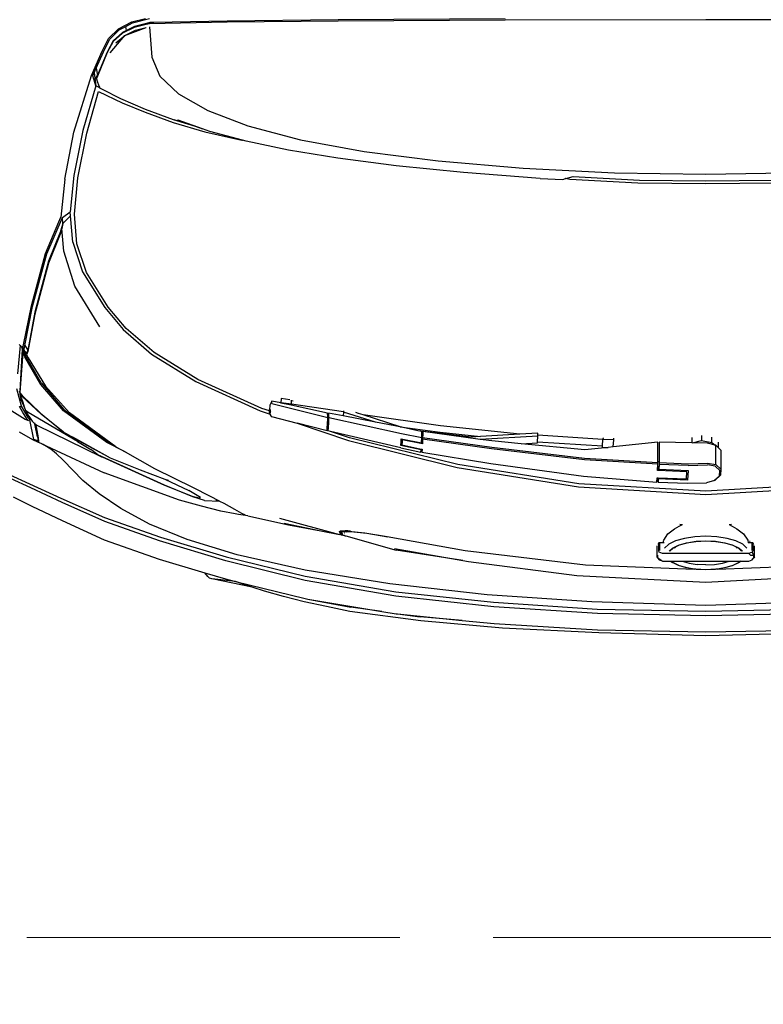
# Model space of a CAD drawing. Units: inches. Extents: x 0 to 4258, y 0 to 3769.
# Tile 6 of 30: x 3739 to 3762, y 2971 to 3003. Entities that reach past the tile are written whole.
import ezdxf

# ---------------------------------------------------------------- set-up
doc = ezdxf.new("R2010")
doc.units = ezdxf.units.IN
doc.header["$MEASUREMENT"] = 0
doc.linetypes.add('ACAD_ISO02W100', pattern=[15, 12, -3])
doc.layers.get('0').update_dxf_attribs({"color": 16})
for name, color, linetype, lineweight in [('A-ANNO-DIMS', 250, 'Continuous', 18), ('A-FLOR-OVHD', 150, 'ACAD_ISO02W100', 13), ('C-PKNG-VEHI', 8, 'Continuous', 18)]:
    doc.layers.add(name, color=color, linetype=linetype, lineweight=lineweight)
doc.layers.add('Edges', color=250, linetype='Continuous')
doc.styles.get("Standard").update_dxf_attribs({"font": 'arial.ttf'})
doc.dimstyles.get("Standard").update_dxf_attribs({"dimtxt": 7, "dimasz": 0.18, "dimexe": 0.18, "dimexo": 0.0625, "dimgap": 0.09, "dimtad": 0, "dimtih": 1, "dimtoh": 1, "dimzin": 0, "dimdsep": 46, "dimlunit": 3, "dimtxsty": 'Standard', "dimcen": 0.09, "dimadec": 0, "dimazin": 0, "dimtfac": 1, "dimtofl": 0, "dimtmove": 0, "dimatfit": 3, "dimfxl": 1, "dimtolj": 1, "dimtzin": 0, "dimarcsym": 0})

# ---------------------------------------------------------------- blocks, each defined once
blk = doc.blocks.new('Nissan Qashqai pl')
at = {"layer": 'Edges'}
for p, q in [((11.05972, 12.11965), (11.05938, 11.92208)), ((11.61327, 11.92208), (11.60675, 12.04892)), ((11.5166, 12.04708), (11.52386, 11.92208)), ((11.52698, 11.92208), (11.51964, 12.0475)), ((11.60051, 11.93346), (11.59629, 12.04057)), ((11.63292, 12.0344), (11.63628, 11.92208)), ((11.64211, 11.92208), (11.63993, 12.02899)), ((11.64437, 12.02886), (11.64655, 11.92208)), ((11.66226, 11.92208), (11.66041, 12.02874)), ((11.66349, 12.02738), (11.66628, 11.92208)), ((11.21164, 11.92208), (11.21014, 12.01197)), ((11.21801, 11.92208), (11.21745, 11.98742)), ((11.22044, 11.98904), (11.22108, 11.92208)), ((11.58846, 11.97008), (11.57758, 11.97008)), ((11.58846, 11.97008), (11.58961, 11.96947)), ((11.56588, 11.95938), (11.57195, 11.96347)), ((11.57195, 11.96347), (11.57457, 11.96395)), ((11.57261, 11.96533), (11.57261, 11.96561)), ((11.57306, 11.96528), (11.57306, 11.96569)), ((11.57479, 11.96843), (11.57457, 11.96768)), ((11.58239, 11.96768), (11.57457, 11.96768)), ((11.57457, 11.96768), (11.57457, 11.96395)), ((11.57457, 11.96395), (11.57457, 11.96378)), ((11.57617, 11.96938), (11.57479, 11.96843)), ((11.57479, 11.96843), (11.58262, 11.96843)), ((11.57994, 11.96265), (11.57613, 11.95845)), ((11.58262, 11.96843), (11.58377, 11.96782)), ((11.58668, 11.96947), (11.58377, 11.96782)), ((11.58377, 11.96782), (11.58513, 11.96453)), ((11.58679, 11.96604), (11.58513, 11.96453)), ((11.58513, 11.96453), (11.58513, 11.87963)), ((11.58679, 11.96604), (11.58668, 11.96947)), ((11.58961, 11.96947), (11.58668, 11.96947)), ((11.5915, 11.96782), (11.58961, 11.96947)), ((11.5915, 11.96782), (11.59043, 11.96839)), ((11.59285, 11.96453), (11.5915, 11.96782)), ((11.59285, 11.95694), (11.59285, 11.96453)), ((11.55816, 11.94815), (11.56082, 11.95281)), ((11.56082, 11.95281), (11.56588, 11.95938)), ((11.57286, 11.95178), (11.57035, 11.94308)), ((11.57613, 11.95845), (11.57286, 11.95178)), ((11.57692, 11.94885), (11.57987, 11.95487)), ((11.57876, 11.95169), (11.57712, 11.94834)), ((11.58001, 11.95424), (11.57876, 11.95169)), ((11.57876, 11.95169), (11.57995, 11.953)), ((11.57987, 11.95487), (11.58291, 11.95821)), ((11.58291, 11.95743), (11.58001, 11.95424)), ((11.59285, 11.95694), (11.59412, 11.95487)), ((11.59285, 11.95657), (11.59285, 11.95694)), ((11.59319, 11.9559), (11.59285, 11.95657)), ((11.59285, 11.95626), (11.59285, 11.95657)), ((11.59285, 11.95626), (11.59319, 11.9559)), ((11.59285, 11.95549), (11.59285, 11.95626)), ((11.59398, 11.95424), (11.59285, 11.95549)), ((11.59285, 11.94526), (11.59285, 11.95549)), ((11.59319, 11.9559), (11.59412, 11.95487)), ((11.59688, 11.94834), (11.59398, 11.95424)), ((11.59412, 11.95487), (11.59707, 11.94885)), ((11.55654, 11.94509), (11.55639, 11.94749)), ((11.55654, 11.94509), (11.55816, 11.94815)), ((11.57035, 11.94308), (11.56877, 11.93295)), ((11.57324, 11.93188), (11.57466, 11.94101)), ((11.57466, 11.94101), (11.57692, 11.94885)), ((11.57712, 11.94834), (11.5749, 11.94065)), ((11.59285, 11.8989), (11.59285, 11.94526)), ((11.59478, 11.93858), (11.59285, 11.94526)), ((11.5991, 11.94065), (11.59688, 11.94834)), ((11.59707, 11.94885), (11.59933, 11.94101)), ((11.59933, 11.94101), (11.60051, 11.93346)), ((11.48106, 11.93457), (11.47554, 11.93456)), ((11.47578, 11.92803), (11.4784, 11.93124)), ((11.4784, 11.93124), (11.47657, 11.92368)), ((11.4786, 11.93206), (11.4784, 11.93124)), ((11.48106, 11.93457), (11.4786, 11.93206)), ((11.49744, 11.93207), (11.4786, 11.93206)), ((11.48349, 11.93703), (11.48106, 11.93457)), ((11.48349, 11.93703), (11.50222, 11.93704)), ((11.49621, 11.92369), (11.49744, 11.93207)), ((11.49744, 11.93207), (11.50222, 11.93704)), ((11.49907, 11.93132), (11.49795, 11.92364)), ((11.50349, 11.93588), (11.49907, 11.93132)), ((11.50222, 11.93704), (11.50812, 11.93671)), ((11.50889, 11.93558), (11.50349, 11.93588)), ((11.50812, 11.93671), (11.51287, 11.9312)), ((11.50889, 11.93558), (11.51321, 11.93053)), ((11.51321, 11.93053), (11.51287, 11.9312)), ((11.56877, 11.93295), (11.56823, 11.92208)), ((11.57275, 11.92208), (11.57324, 11.93188)), ((11.5735, 11.93169), (11.57302, 11.92208)), ((11.5749, 11.94065), (11.5735, 11.93169)), ((11.59602, 11.93062), (11.59478, 11.93858)), ((11.60049, 11.93169), (11.5991, 11.94065)), ((11.60097, 11.92208), (11.60049, 11.93169)), ((11.60051, 11.93346), (11.60076, 11.93188)), ((11.60076, 11.93188), (11.60124, 11.92208)), ((11.05938, 11.92208), (11.05972, 11.72451)), ((11.21014, 11.8322), (11.21164, 11.92208)), ((11.21745, 11.85674), (11.21801, 11.92208)), ((11.22108, 11.92208), (11.22044, 11.85512)), ((11.47578, 11.92803), (11.47062, 11.92803)), ((11.47398, 11.91798), (11.47578, 11.92803)), ((11.47657, 11.92368), (11.47622, 11.90912)), ((11.49689, 11.90495), (11.49621, 11.92369)), ((11.49859, 11.9049), (11.49795, 11.92364)), ((11.51321, 11.93053), (11.51543, 11.92267)), ((11.51606, 11.90392), (11.51543, 11.92267)), ((11.52386, 11.92208), (11.5166, 11.79708)), ((11.51964, 11.79666), (11.52698, 11.92208)), ((11.56823, 11.92208), (11.56877, 11.91121)), ((11.57324, 11.91228), (11.57275, 11.92208)), ((11.57302, 11.92208), (11.5735, 11.91247)), ((11.59645, 11.92208), (11.59602, 11.93062)), ((11.59645, 11.92208), (11.59602, 11.91354)), ((11.60049, 11.91247), (11.60097, 11.92208)), ((11.60124, 11.92208), (11.60076, 11.91228)), ((11.60675, 11.79524), (11.61327, 11.92208)), ((11.63628, 11.92208), (11.63292, 11.80976)), ((11.63993, 11.81518), (11.64211, 11.92208)), ((11.64655, 11.92208), (11.64437, 11.8153)), ((11.66041, 11.81542), (11.66226, 11.92208)), ((11.66628, 11.92208), (11.66349, 11.81678)), ((11.46896, 11.91798), (11.47398, 11.91798)), ((11.47622, 11.90912), (11.47398, 11.91798)), ((11.57466, 11.90315), (11.57324, 11.91228)), ((11.5735, 11.91247), (11.5749, 11.90351)), ((11.59478, 11.90558), (11.59602, 11.91354)), ((11.5991, 11.90351), (11.60049, 11.91247)), ((11.60076, 11.91228), (11.60051, 11.91071)), ((11.47102, 11.90825), (11.4762, 11.90826)), ((11.4762, 11.90826), (11.47542, 11.87608)), ((11.47622, 11.90912), (11.4762, 11.90826)), ((11.49565, 11.87616), (11.49689, 11.90495)), ((11.49859, 11.9049), (11.49735, 11.87612)), ((11.50223, 11.8759), (11.50346, 11.90468)), ((11.50462, 11.90341), (11.50341, 11.87505)), ((11.50346, 11.90468), (11.51299, 11.90415)), ((11.51177, 11.90301), (11.50462, 11.90341)), ((11.51058, 11.87508), (11.51177, 11.90301)), ((11.51299, 11.90415), (11.51176, 11.87537)), ((11.51483, 11.87514), (11.51606, 11.90392)), ((11.56877, 11.91121), (11.57035, 11.90108)), ((11.57692, 11.89531), (11.57466, 11.90315)), ((11.5749, 11.90351), (11.57712, 11.89582)), ((11.59285, 11.8989), (11.59478, 11.90558)), ((11.59629, 11.80359), (11.60051, 11.91071)), ((11.59688, 11.89582), (11.5991, 11.90351)), ((11.59933, 11.90315), (11.59707, 11.89531)), ((11.60051, 11.91071), (11.59933, 11.90315)), ((11.55639, 11.89667), (11.55654, 11.89907)), ((11.55816, 11.89601), (11.55654, 11.89907)), ((11.56082, 11.89135), (11.55816, 11.89601)), ((11.57035, 11.90108), (11.57286, 11.89238)), ((11.57286, 11.89238), (11.57613, 11.88571)), ((11.57987, 11.88929), (11.57692, 11.89531)), ((11.57712, 11.89582), (11.57876, 11.89248)), ((11.57995, 11.89116), (11.57876, 11.89248)), ((11.57876, 11.89248), (11.58001, 11.88992)), ((11.59285, 11.88868), (11.59285, 11.8989)), ((11.59398, 11.88992), (11.59688, 11.89582)), ((11.59707, 11.89531), (11.59412, 11.88929)), ((11.56588, 11.88478), (11.56082, 11.89135)), ((11.57195, 11.88069), (11.56588, 11.88478)), ((11.57613, 11.88571), (11.57994, 11.88151)), ((11.58291, 11.88595), (11.57987, 11.88929)), ((11.58001, 11.88992), (11.58291, 11.88673)), ((11.59285, 11.88868), (11.59398, 11.88992)), ((11.59285, 11.88722), (11.59412, 11.88929)), ((11.59285, 11.8879), (11.59285, 11.88868)), ((11.59285, 11.88759), (11.59319, 11.88827)), ((11.59319, 11.88827), (11.59285, 11.8879)), ((11.59285, 11.88759), (11.59285, 11.8879)), ((11.59285, 11.88722), (11.59285, 11.88759)), ((11.59285, 11.87963), (11.59285, 11.88722)), ((11.59412, 11.88929), (11.59319, 11.88827)), ((11.49563, 11.87496), (11.47539, 11.87488)), ((11.47539, 11.87488), (11.4801, 11.83099)), ((11.47542, 11.87608), (11.49451, 11.87616)), ((11.49133, 11.80278), (11.49563, 11.87496)), ((11.49732, 11.87492), (11.49295, 11.80271)), ((11.49449, 11.87502), (11.49451, 11.87616)), ((11.50341, 11.87505), (11.49449, 11.87502)), ((11.49451, 11.87616), (11.49565, 11.87616)), ((11.49732, 11.87492), (11.49563, 11.87496)), ((11.49565, 11.87616), (11.49735, 11.87612)), ((11.50339, 11.87463), (11.49732, 11.87492)), ((11.49735, 11.87612), (11.50223, 11.8759)), ((11.50341, 11.87505), (11.50339, 11.87463)), ((11.50884, 11.80182), (11.5148, 11.87394)), ((11.51054, 11.87423), (11.51058, 11.87508)), ((11.5148, 11.87394), (11.51054, 11.87423)), ((11.51472, 11.8751), (11.51058, 11.87508)), ((11.51176, 11.87537), (11.51472, 11.87515)), ((11.51472, 11.87515), (11.51472, 11.8751)), ((11.51472, 11.87515), (11.51483, 11.87514)), ((11.51483, 11.87514), (11.51472, 11.8751)), ((11.57261, 11.88057), (11.57195, 11.88069)), ((11.57261, 11.88057), (11.57261, 11.88076)), ((11.57306, 11.88049), (11.57261, 11.88057)), ((11.57306, 11.88049), (11.57306, 11.88081)), ((11.57457, 11.88021), (11.57306, 11.88049)), ((11.57457, 11.88096), (11.57457, 11.88021)), ((11.57457, 11.88021), (11.57457, 11.87648)), ((11.57457, 11.87648), (11.58239, 11.87648)), ((11.57457, 11.87648), (11.57479, 11.87573)), ((11.58262, 11.87573), (11.57479, 11.87573)), ((11.57479, 11.87573), (11.57617, 11.87478)), ((11.58846, 11.87408), (11.57758, 11.87408)), ((11.58377, 11.87635), (11.58262, 11.87573)), ((11.58513, 11.87963), (11.58377, 11.87635)), ((11.58668, 11.87469), (11.58961, 11.87469)), ((11.58961, 11.87469), (11.58846, 11.87408)), ((11.58961, 11.87469), (11.5915, 11.87635)), ((11.59043, 11.87577), (11.58961, 11.87469)), ((11.59221, 11.87812), (11.59043, 11.87577)), ((11.59043, 11.87577), (11.5915, 11.87635)), ((11.5915, 11.87635), (11.59221, 11.87812)), ((11.59285, 11.87963), (11.59221, 11.87812)), ((11.2139, 11.7914), (11.21745, 11.85674)), ((11.22044, 11.85512), (11.21682, 11.78816)), ((11.20565, 11.74231), (11.21014, 11.8322)), ((11.47305, 11.83139), (11.47165, 11.83144)), ((11.47305, 11.83139), (11.473, 11.82087)), ((11.4801, 11.83099), (11.47305, 11.83139)), ((11.4801, 11.83099), (11.48065, 11.82584)), ((11.48062, 11.82044), (11.48065, 11.82584)), ((11.48065, 11.82584), (11.4831, 11.803)), ((11.47281, 11.82086), (11.46872, 11.75675)), ((11.47111, 11.82093), (11.47189, 11.82089)), ((11.47281, 11.82086), (11.47189, 11.82089)), ((11.473, 11.82087), (11.47281, 11.82086)), ((11.47916, 11.8205), (11.473, 11.82087)), ((11.47508, 11.75641), (11.47919, 11.82046)), ((11.47919, 11.82046), (11.47916, 11.8205)), ((11.48062, 11.82044), (11.47919, 11.82046)), ((11.63327, 11.71316), (11.63993, 11.81518)), ((11.64437, 11.8153), (11.63768, 11.7134)), ((11.65425, 11.71357), (11.66041, 11.81542)), ((11.66349, 11.81678), (11.65888, 11.72193)), ((11.63292, 11.80976), (11.62604, 11.70665)), ((11.4831, 11.803), (11.47707, 11.74042)), ((11.4805, 11.71128), (11.49133, 11.80278)), ((11.49295, 11.80271), (11.48212, 11.71121)), ((11.49642, 11.71041), (11.50884, 11.80182)), ((11.5166, 11.79708), (11.49761, 11.67796)), ((11.50045, 11.6772), (11.51964, 11.79666)), ((11.58235, 11.68521), (11.59629, 11.80359)), ((11.21579, 11.78424), (11.2139, 11.7914)), ((11.21682, 11.78816), (11.21579, 11.78424)), ((11.21682, 11.78816), (11.21585, 11.78401)), ((11.5932, 11.68852), (11.60675, 11.79524)), ((11.21585, 11.78401), (11.21579, 11.78424)), ((11.21658, 11.78121), (11.21585, 11.78401)), ((11.21586, 11.75915), (11.21658, 11.78121)), ((11.21586, 11.75915), (11.20997, 11.68347)), ((11.46872, 11.75675), (11.46649, 11.75682)), ((11.46649, 11.75682), (11.46757, 11.73891)), ((11.46975, 11.75671), (11.46872, 11.75675)), ((11.46975, 11.75671), (11.47273, 11.69994)), ((11.47508, 11.75641), (11.46975, 11.75671)), ((11.47611, 11.75636), (11.47508, 11.75641)), ((11.47707, 11.74042), (11.47611, 11.75636)), ((11.19842, 11.65867), (11.20565, 11.74231)), ((11.46757, 11.73891), (11.45941, 11.6607)), ((11.46757, 11.73891), (11.46992, 11.70014)), ((11.47707, 11.74042), (11.47428, 11.71144)), ((11.0586, 11.72441), (11.05947, 11.55994)), ((11.05972, 11.72451), (11.06059, 11.56009)), ((11.65888, 11.72193), (11.65143, 11.64152)), ((11.47094, 11.64327), (11.4805, 11.71128)), ((11.48212, 11.71121), (11.47257, 11.6432)), ((11.47428, 11.71144), (11.47273, 11.69994)), ((11.48539, 11.64249), (11.49642, 11.71041)), ((11.6229, 11.61679), (11.63327, 11.71316)), ((11.63768, 11.7134), (11.62719, 11.61693)), ((11.65114, 11.68233), (11.65425, 11.71357)), ((11.47273, 11.69994), (11.46512, 11.64343)), ((11.46576, 11.66035), (11.46992, 11.70014)), ((11.46992, 11.70014), (11.47047, 11.69095)), ((11.62604, 11.70665), (11.61495, 11.61084)), ((11.47047, 11.69095), (11.46419, 11.63849)), ((11.20997, 11.68347), (11.2033, 11.61723)), ((11.56846, 11.60829), (11.58235, 11.68521)), ((11.58021, 11.61555), (11.59218, 11.68277)), ((11.59218, 11.68277), (11.58179, 11.61717)), ((11.59218, 11.68277), (11.5932, 11.68852)), ((11.64478, 11.61839), (11.65114, 11.68233)), ((11.65114, 11.68233), (11.64749, 11.64092)), ((11.49761, 11.67796), (11.47115, 11.57128)), ((11.47375, 11.5702), (11.50045, 11.6772)), ((11.45941, 11.6607), (11.44866, 11.58459)), ((11.46024, 11.62121), (11.46576, 11.66035)), ((11.18907, 11.58559), (11.19842, 11.65867)), ((11.46505, 11.64255), (11.46419, 11.63849)), ((11.46792, 11.64248), (11.46505, 11.64255)), ((11.46512, 11.64343), (11.46801, 11.64335)), ((11.46687, 11.62247), (11.47088, 11.64239)), ((11.46801, 11.64335), (11.46792, 11.64248)), ((11.47088, 11.64239), (11.46792, 11.64248)), ((11.46801, 11.64335), (11.47094, 11.64327)), ((11.47252, 11.64233), (11.47088, 11.64239)), ((11.47094, 11.64327), (11.47257, 11.6432)), ((11.47212, 11.62223), (11.47625, 11.64214)), ((11.47439, 11.64223), (11.47252, 11.64233)), ((11.47257, 11.6432), (11.47449, 11.6431)), ((11.47727, 11.64296), (11.47315, 11.62305)), ((11.47439, 11.64223), (11.47449, 11.6431)), ((11.47625, 11.64214), (11.47439, 11.64223)), ((11.47449, 11.6431), (11.47727, 11.64296)), ((11.47827, 11.62277), (11.48226, 11.64167)), ((11.48298, 11.64165), (11.47879, 11.62186)), ((11.48098, 11.62171), (11.48532, 11.64161)), ((11.48226, 11.64167), (11.48244, 11.64254)), ((11.48226, 11.64167), (11.48298, 11.64165)), ((11.48244, 11.64254), (11.48247, 11.64267)), ((11.48535, 11.64246), (11.48244, 11.64254)), ((11.48247, 11.64267), (11.48535, 11.64246)), ((11.483, 11.64176), (11.48298, 11.64165)), ((11.48532, 11.64161), (11.483, 11.64176)), ((11.48539, 11.64249), (11.48535, 11.64246)), ((11.65143, 11.64152), (11.64217, 11.57162)), ((11.64478, 11.61839), (11.64749, 11.64092)), ((11.46419, 11.63849), (11.46114, 11.62406)), ((11.46024, 11.62121), (11.44866, 11.58459)), ((11.45125, 11.55073), (11.46687, 11.62247)), ((11.46083, 11.62261), (11.45585, 11.5969)), ((11.46114, 11.62406), (11.46024, 11.62121)), ((11.46114, 11.62406), (11.46083, 11.62261)), ((11.48098, 11.62171), (11.4649, 11.55261)), ((11.47495, 11.62207), (11.47212, 11.62223)), ((11.47315, 11.62305), (11.47515, 11.62294)), ((11.47495, 11.62207), (11.47515, 11.62294)), ((11.47879, 11.62186), (11.47495, 11.62207)), ((11.47515, 11.62294), (11.47827, 11.62277)), ((11.2033, 11.61723), (11.19582, 11.55976)), ((11.56776, 11.56755), (11.58179, 11.61717)), ((11.60765, 11.5276), (11.6229, 11.61679)), ((11.62719, 11.61693), (11.61178, 11.52762)), ((11.64227, 11.603), (11.64462, 11.61709)), ((11.64462, 11.61709), (11.64478, 11.61839)), ((11.56499, 11.58644), (11.56846, 11.60829)), ((11.56905, 11.60888), (11.56563, 11.58822)), ((11.61495, 11.61084), (11.6016, 11.52761)), ((11.63012, 11.53004), (11.64227, 11.603)), ((11.64227, 11.603), (11.63807, 11.5726)), ((11.45585, 11.5969), (11.44582, 11.56516)), ((11.45585, 11.5969), (11.44965, 11.56495)), ((11.17758, 11.52307), (11.18907, 11.58559)), ((11.44866, 11.58459), (11.44723, 11.58007)), ((11.56356, 11.57357), (11.56499, 11.58644)), ((11.56563, 11.58822), (11.56415, 11.57536)), ((11.44723, 11.58007), (11.44639, 11.57739)), ((11.56335, 11.56843), (11.56356, 11.57357)), ((11.56415, 11.57536), (11.56375, 11.56794)), ((11.63012, 11.53004), (11.63807, 11.5726)), ((11.44575, 11.56516), (11.43801, 11.51398)), ((11.4448, 11.5652), (11.44575, 11.56516)), ((11.44575, 11.56516), (11.44582, 11.56516)), ((11.44582, 11.56516), (11.44965, 11.56495)), ((11.44965, 11.56495), (11.44685, 11.5505)), ((11.45676, 11.51971), (11.47375, 11.5702)), ((11.47115, 11.57128), (11.4649, 11.55261)), ((11.56255, 11.56701), (11.56268, 11.56956)), ((11.56271, 11.56245), (11.56255, 11.56701)), ((11.56268, 11.56956), (11.56259, 11.5697)), ((11.56268, 11.56956), (11.5628, 11.57206)), ((11.56335, 11.56843), (11.56268, 11.56956)), ((11.56334, 11.56271), (11.56271, 11.56245)), ((11.56325, 11.56586), (11.56335, 11.56843)), ((11.56334, 11.56271), (11.56325, 11.56586)), ((11.56609, 11.56386), (11.56334, 11.56271)), ((11.56338, 11.56129), (11.56334, 11.56271)), ((11.56368, 11.56788), (11.56335, 11.56843)), ((11.56375, 11.56794), (11.56392, 11.56325)), ((11.56392, 11.56325), (11.56429, 11.56338)), ((11.56429, 11.56338), (11.56596, 11.56408)), ((11.56487, 11.5659), (11.56469, 11.5662)), ((11.56609, 11.56386), (11.56583, 11.56223)), ((11.56596, 11.56408), (11.56616, 11.56417)), ((11.56609, 11.56386), (11.56596, 11.56408)), ((11.56613, 11.56388), (11.56609, 11.56386)), ((11.56618, 11.56418), (11.56613, 11.56388)), ((11.56613, 11.56388), (11.56616, 11.56417)), ((11.56613, 11.56388), (11.56645, 11.5641)), ((11.56665, 11.56424), (11.56616, 11.56236)), ((11.56616, 11.56417), (11.56618, 11.56418)), ((11.56616, 11.56236), (11.56645, 11.5641)), ((11.56618, 11.56418), (11.56648, 11.56431)), ((11.56645, 11.5641), (11.56648, 11.56431)), ((11.56645, 11.5641), (11.56665, 11.56424)), ((11.56648, 11.56431), (11.56669, 11.5644)), ((11.56679, 11.56261), (11.56648, 11.56144)), ((11.56661, 11.56253), (11.56704, 11.56455)), ((11.56671, 11.56257), (11.56661, 11.56253)), ((11.56665, 11.56424), (11.56688, 11.56448)), ((11.56669, 11.5644), (11.56665, 11.56424)), ((11.56669, 11.5644), (11.56688, 11.56448)), ((11.56671, 11.56257), (11.56712, 11.56458)), ((11.56679, 11.56261), (11.56671, 11.56257)), ((11.56717, 11.5646), (11.56679, 11.56261)), ((11.56688, 11.56448), (11.56704, 11.56455)), ((11.56704, 11.56455), (11.56739, 11.56625)), ((11.56704, 11.56455), (11.56712, 11.56458)), ((11.56712, 11.56458), (11.56763, 11.56708)), ((11.56712, 11.56458), (11.56717, 11.5646)), ((11.56717, 11.5646), (11.56763, 11.56708)), ((11.56745, 11.56646), (11.56739, 11.56625)), ((11.56763, 11.56708), (11.56776, 11.56755)), ((11.64217, 11.57162), (11.63751, 11.54857)), ((11.05947, 11.55994), (11.06074, 11.45082)), ((11.06059, 11.56009), (11.06182, 11.4509)), ((11.19582, 11.55976), (11.18773, 11.51111)), ((11.55053, 11.5023), (11.56648, 11.56144)), ((11.56338, 11.56129), (11.56271, 11.56245)), ((11.56273, 11.5431), (11.56648, 11.56144)), ((11.56583, 11.56223), (11.56338, 11.56129)), ((11.56616, 11.56236), (11.56583, 11.56223)), ((11.56661, 11.56253), (11.56616, 11.56236)), ((11.43747, 11.49463), (11.45125, 11.54985)), ((11.44684, 11.54963), (11.43914, 11.51392)), ((11.44983, 11.54978), (11.44684, 11.54963)), ((11.44685, 11.5505), (11.44997, 11.55066)), ((11.44983, 11.54978), (11.44997, 11.55066)), ((11.45125, 11.54985), (11.44983, 11.54978)), ((11.44997, 11.55066), (11.45125, 11.55073)), ((11.45125, 11.55073), (11.4529, 11.55066)), ((11.4529, 11.54978), (11.45125, 11.54985)), ((11.4529, 11.55066), (11.45711, 11.55045)), ((11.45711, 11.54958), (11.4529, 11.54978)), ((11.46429, 11.54915), (11.45676, 11.51971)), ((11.45711, 11.55045), (11.45994, 11.5503)), ((11.46197, 11.5493), (11.45711, 11.54958)), ((11.45983, 11.54978), (11.45994, 11.5503)), ((11.46402, 11.54999), (11.45983, 11.54978)), ((11.45994, 11.5503), (11.46197, 11.55018)), ((11.46197, 11.55018), (11.46404, 11.55004)), ((11.46375, 11.54918), (11.46197, 11.5493)), ((11.46402, 11.54999), (11.46375, 11.54918)), ((11.46429, 11.54915), (11.46375, 11.54918)), ((11.46404, 11.55004), (11.46402, 11.54999)), ((11.46423, 11.55), (11.46402, 11.54999)), ((11.46404, 11.55004), (11.46423, 11.55)), ((11.46423, 11.55), (11.46424, 11.55003)), ((11.4643, 11.55002), (11.46423, 11.55)), ((11.4649, 11.55261), (11.4643, 11.55002)), ((11.63751, 11.54857), (11.63276, 11.52672)), ((11.55533, 11.50682), (11.56273, 11.5431)), ((11.55707, 11.51104), (11.56273, 11.5431)), ((11.6016, 11.52761), (11.58664, 11.46068)), ((11.58843, 11.44985), (11.60765, 11.5276)), ((11.61178, 11.52762), (11.59225, 11.44945)), ((11.61272, 11.45895), (11.62966, 11.52759)), ((11.63276, 11.52672), (11.62771, 11.50627)), ((11.62966, 11.52759), (11.63012, 11.53004)), ((11.16395, 11.47112), (11.17758, 11.52307)), ((11.43475, 11.51409), (11.43403, 11.51411)), ((11.43501, 11.51584), (11.43475, 11.51409)), ((11.43801, 11.51398), (11.43475, 11.51409)), ((11.45032, 11.49453), (11.45676, 11.51971)), ((11.18773, 11.51111), (11.17906, 11.46956)), ((11.43371, 11.51238), (11.43251, 11.50378)), ((11.4382, 11.51397), (11.43676, 11.50364)), ((11.43914, 11.51392), (11.43692, 11.50363)), ((11.4382, 11.51397), (11.43801, 11.51398)), ((11.43914, 11.51392), (11.4382, 11.51397)), ((11.54814, 11.47101), (11.55707, 11.51104)), ((11.62771, 11.50627), (11.62241, 11.48743)), ((11.43251, 11.50378), (11.43676, 11.50364)), ((11.43251, 11.50378), (11.4369, 11.50353)), ((11.4369, 11.50353), (11.435, 11.49469)), ((11.435, 11.49469), (11.43896, 11.49272)), ((11.43747, 11.49463), (11.435, 11.49469)), ((11.43676, 11.50364), (11.43692, 11.50363)), ((11.43692, 11.50363), (11.4369, 11.50353)), ((11.43896, 11.49272), (11.44373, 11.49245)), ((11.44474, 11.49242), (11.44218, 11.48476)), ((11.44507, 11.49341), (11.44316, 11.49351)), ((11.44373, 11.49245), (11.44491, 11.49291)), ((11.44474, 11.49242), (11.44373, 11.49245)), ((11.44453, 11.48334), (11.44778, 11.49299)), ((11.44491, 11.49291), (11.44474, 11.49242)), ((11.4462, 11.49239), (11.44474, 11.49242)), ((11.44507, 11.49341), (11.44491, 11.49291)), ((11.44491, 11.49291), (11.44606, 11.49335)), ((11.44606, 11.49335), (11.44507, 11.49341)), ((11.44786, 11.49325), (11.44606, 11.49335)), ((11.44786, 11.49325), (11.4462, 11.49239)), ((11.44778, 11.49299), (11.4462, 11.49239)), ((11.45018, 11.49392), (11.44778, 11.49299)), ((11.44794, 11.49325), (11.44786, 11.49325)), ((11.45032, 11.49453), (11.44794, 11.49325)), ((11.45018, 11.49392), (11.45032, 11.49453)), ((11.62241, 11.48743), (11.61848, 11.47528)), ((11.44218, 11.48476), (11.41383, 11.42186)), ((11.41588, 11.41997), (11.44453, 11.48334)), ((11.61848, 11.47528), (11.61008, 11.43562)), ((11.61848, 11.47528), (11.61742, 11.47198)), ((11.14869, 11.43161), (11.16395, 11.47112)), ((11.17808, 11.46592), (11.1694, 11.43374)), ((11.17797, 11.4652), (11.17808, 11.46592)), ((11.17906, 11.46956), (11.17808, 11.46592)), ((11.54554, 11.46484), (11.54721, 11.46841)), ((11.54814, 11.47101), (11.54666, 11.46197)), ((11.61742, 11.47198), (11.61272, 11.45895)), ((11.1699, 11.42889), (11.17797, 11.4652)), ((11.53572, 11.44731), (11.54162, 11.45783)), ((11.54162, 11.45783), (11.54554, 11.46484)), ((11.54611, 11.45874), (11.54336, 11.44449)), ((11.54666, 11.46197), (11.54611, 11.45874)), ((11.58664, 11.46068), (11.57152, 11.41151)), ((11.61272, 11.45895), (11.61008, 11.43562)), ((11.61028, 11.44915), (11.61272, 11.45895)), ((11.06074, 11.45082), (11.06214, 11.37845)), ((11.06182, 11.4509), (11.06324, 11.37414)), ((11.53354, 11.44315), (11.53572, 11.44731)), ((11.56912, 11.38501), (11.58843, 11.44985)), ((11.59225, 11.44945), (11.57263, 11.38419)), ((11.60419, 11.42861), (11.61028, 11.44915)), ((11.52833, 11.43321), (11.53335, 11.4428)), ((11.53261, 11.43965), (11.5333, 11.44225)), ((11.53313, 11.42848), (11.53354, 11.44315)), ((11.5333, 11.44225), (11.53335, 11.4428)), ((11.53335, 11.4428), (11.53354, 11.44315)), ((11.54336, 11.44449), (11.53855, 11.42543)), ((11.1323, 11.40268), (11.14869, 11.43161)), ((11.16047, 11.39766), (11.1699, 11.42889)), ((11.1694, 11.43374), (11.1668, 11.42651)), ((11.5202, 11.41712), (11.52833, 11.43321)), ((11.53313, 11.42848), (11.52922, 11.417)), ((11.59084, 11.38361), (11.60419, 11.42861)), ((11.60772, 11.43162), (11.60419, 11.42861)), ((11.60938, 11.43347), (11.60772, 11.43162)), ((11.61008, 11.43562), (11.60938, 11.43347)), ((11.15764, 11.39828), (11.16426, 11.41918)), ((11.15766, 11.39771), (11.16426, 11.41918)), ((11.1668, 11.42651), (11.1582, 11.40259)), ((11.16426, 11.41918), (11.15826, 11.40186)), ((11.16426, 11.41918), (11.1668, 11.42651)), ((11.41383, 11.42186), (11.38718, 11.37878)), ((11.38877, 11.37638), (11.41588, 11.41997)), ((11.50131, 11.37908), (11.5202, 11.41712)), ((11.53009, 11.42439), (11.52299, 11.41307)), ((11.52855, 11.41625), (11.53022, 11.42324)), ((11.53022, 11.42324), (11.53009, 11.42439)), ((11.53855, 11.42543), (11.53253, 11.4038)), ((11.5118, 11.38938), (11.52299, 11.41307)), ((11.52922, 11.417), (11.51787, 11.38901)), ((11.51787, 11.38901), (11.52855, 11.41625)), ((11.57152, 11.41151), (11.55624, 11.37411)), ((11.11477, 11.38434), (11.1323, 11.40268)), ((11.14751, 11.37001), (11.15766, 11.39771)), ((11.15051, 11.36998), (11.16047, 11.39766)), ((11.53253, 11.4038), (11.50574, 11.32965)), ((11.51787, 11.38901), (11.48801, 11.32337)), ((11.49005, 11.3275), (11.51787, 11.38901)), ((11.50277, 11.36495), (11.5118, 11.38938)), ((11.5118, 11.38938), (11.51304, 11.39274)), ((11.06214, 11.37845), (11.06222, 11.37449)), ((11.09618, 11.37663), (11.11477, 11.38434)), ((11.38718, 11.37878), (11.3635, 11.35125)), ((11.48518, 11.35017), (11.50131, 11.37908)), ((11.54963, 11.33002), (11.56912, 11.38501)), ((11.57263, 11.38419), (11.5535, 11.33028)), ((11.57164, 11.32969), (11.59084, 11.38361)), ((11.06139, 11.35691), (11.05807, 11.37037)), ((11.06236, 11.3576), (11.05822, 11.37418)), ((11.06222, 11.37449), (11.06303, 11.37135)), ((11.06303, 11.37135), (11.06594, 11.3594)), ((11.06324, 11.37414), (11.06408, 11.37085)), ((11.06408, 11.37085), (11.06692, 11.35921)), ((11.06624, 11.37435), (11.09618, 11.37663)), ((11.06961, 11.36056), (11.0671, 11.37109)), ((11.07472, 11.34981), (11.0671, 11.37109)), ((11.13692, 11.34555), (11.14751, 11.37001)), ((11.14123, 11.34726), (11.15051, 11.36998)), ((11.36451, 11.34835), (11.38877, 11.37638)), ((11.55624, 11.37411), (11.54097, 11.34593)), ((11.06594, 11.3594), (11.06978, 11.35164)), ((11.06692, 11.35921), (11.0727, 11.34754)), ((11.07472, 11.34981), (11.06961, 11.36056)), ((11.49086, 11.33567), (11.50277, 11.36495)), ((11.06818, 11.34377), (11.06139, 11.35691)), ((11.06584, 11.35092), (11.06236, 11.3576)), ((11.06978, 11.35164), (11.06584, 11.35092)), ((11.06918, 11.34452), (11.06584, 11.35092)), ((11.06978, 11.35164), (11.07183, 11.3475)), ((11.08206, 11.34125), (11.07472, 11.34981)), ((11.092, 11.33548), (11.07472, 11.34981)), ((11.3635, 11.35125), (11.34251, 11.3336)), ((11.48518, 11.35017), (11.4758, 11.33232)), ((11.48012, 11.34111), (11.48518, 11.35017)), ((11.07787, 11.3339), (11.06818, 11.34377)), ((11.07866, 11.33492), (11.06918, 11.34452)), ((11.07183, 11.3475), (11.08018, 11.33842)), ((11.0727, 11.34754), (11.0809, 11.33858)), ((11.12767, 11.32749), (11.13692, 11.34555)), ((11.13017, 11.32416), (11.14123, 11.34726)), ((11.34283, 11.33026), (11.36451, 11.34835)), ((11.48005, 11.341), (11.44669, 11.29536)), ((11.47876, 11.33901), (11.48005, 11.341)), ((11.48005, 11.341), (11.48012, 11.34111)), ((11.54097, 11.34593), (11.52646, 11.32473)), ((11.09022, 11.32753), (11.07787, 11.3339)), ((11.09081, 11.32882), (11.07866, 11.33492)), ((11.08018, 11.33842), (11.09121, 11.33249)), ((11.0809, 11.33858), (11.09174, 11.33271)), ((11.09121, 11.33249), (11.1138, 11.3229)), ((11.09174, 11.33271), (11.11486, 11.323)), ((11.30757, 11.30833), (11.34283, 11.33026)), ((11.34251, 11.3336), (11.3082, 11.31215)), ((11.44331, 11.28988), (11.47454, 11.33252)), ((11.4758, 11.33232), (11.44474, 11.28965)), ((11.46332, 11.28473), (11.48966, 11.33337)), ((11.47038, 11.29841), (11.49086, 11.33567)), ((11.47038, 11.29841), (11.48966, 11.33337)), ((11.47876, 11.33901), (11.47454, 11.33252)), ((11.48966, 11.33337), (11.49086, 11.33567)), ((11.53062, 11.28691), (11.54963, 11.33002)), ((11.5535, 11.33028), (11.53487, 11.28826)), ((11.11439, 11.31711), (11.09022, 11.32753)), ((11.10704, 11.32181), (11.09081, 11.32882)), ((11.10704, 11.32181), (11.1138, 11.3229)), ((11.11164, 11.31982), (11.10704, 11.32181)), ((11.11164, 11.31982), (11.1244, 11.32146)), ((11.1138, 11.3229), (11.11393, 11.32284)), ((11.11393, 11.32284), (11.1164, 11.32172)), ((11.1244, 11.32146), (11.11467, 11.31851)), ((11.11486, 11.323), (11.1172, 11.32196)), ((11.1164, 11.32172), (11.1172, 11.32196)), ((11.11744, 11.32189), (11.1164, 11.32172)), ((11.1172, 11.32196), (11.11744, 11.32189)), ((11.11744, 11.32189), (11.11997, 11.32267)), ((11.11997, 11.32267), (11.12459, 11.32429)), ((11.12604, 11.32481), (11.1244, 11.32146)), ((11.1244, 11.32146), (11.12591, 11.32476)), ((11.1244, 11.32146), (11.16836, 11.30873)), ((11.12459, 11.32429), (11.12591, 11.32476)), ((11.12466, 11.32442), (11.12595, 11.32486)), ((11.12478, 11.32467), (11.12595, 11.32486)), ((11.12595, 11.32486), (11.1251, 11.3253)), ((11.12591, 11.32476), (11.12595, 11.32486)), ((11.12591, 11.32476), (11.12604, 11.32481)), ((11.12595, 11.32486), (11.12626, 11.32554)), ((11.12595, 11.32486), (11.12607, 11.32488)), ((11.12604, 11.32481), (11.12645, 11.32495)), ((11.12607, 11.32488), (11.12604, 11.32481)), ((11.12631, 11.32537), (11.12607, 11.32488)), ((11.12607, 11.32488), (11.12645, 11.32495)), ((11.12645, 11.32495), (11.12767, 11.32749)), ((11.17121, 11.31245), (11.13017, 11.32416)), ((11.36192, 11.32544), (11.32179, 11.30083)), ((11.45883, 11.26345), (11.48954, 11.32636)), ((11.48133, 11.27727), (11.50574, 11.32965)), ((11.48801, 11.32337), (11.48281, 11.31653)), ((11.48983, 11.32694), (11.48954, 11.32636)), ((11.48983, 11.32694), (11.49005, 11.3275)), ((11.52646, 11.32473), (11.51313, 11.30854)), ((11.55274, 11.28821), (11.57164, 11.32969)), ((11.11467, 11.31851), (11.11164, 11.31982)), ((11.17021, 11.29978), (11.11439, 11.31711)), ((11.21523, 11.3038), (11.17121, 11.31245)), ((11.3082, 11.31215), (11.28005, 11.30276)), ((11.47499, 11.30324), (11.48281, 11.31653)), ((11.16836, 11.30873), (11.21271, 11.29983)), ((11.2509, 11.3003), (11.21523, 11.3038)), ((11.28005, 11.30276), (11.2509, 11.3003)), ((11.27848, 11.29865), (11.30757, 11.30833)), ((11.32179, 11.30083), (11.28736, 11.28974)), ((11.47499, 11.30324), (11.4462, 11.25482)), ((11.51313, 11.30854), (11.49329, 11.28912)), ((11.21656, 11.2908), (11.17021, 11.29978)), ((11.21271, 11.29983), (11.24875, 11.29618)), ((11.25238, 11.29648), (11.24875, 11.29618)), ((11.2541, 11.28846), (11.24875, 11.29618)), ((11.27848, 11.29865), (11.25238, 11.29648)), ((11.25238, 11.29648), (11.25993, 11.28891)), ((11.42028, 11.27173), (11.44669, 11.29536)), ((11.46587, 11.29022), (11.46737, 11.29293)), ((11.46746, 11.29312), (11.46737, 11.29293)), ((11.46746, 11.29312), (11.47026, 11.29821)), ((11.47026, 11.29821), (11.47038, 11.29841)), ((11.21656, 11.2908), (11.25377, 11.28706)), ((11.25857, 11.28503), (11.25377, 11.28706)), ((11.25993, 11.28891), (11.2541, 11.28846)), ((11.29, 11.2731), (11.2541, 11.28846)), ((11.28951, 11.27177), (11.25857, 11.28503)), ((11.25993, 11.28891), (11.25999, 11.28889)), ((11.25999, 11.28889), (11.26503, 11.28789)), ((11.25999, 11.28889), (11.26771, 11.28668)), ((11.27242, 11.28847), (11.26503, 11.28789)), ((11.26503, 11.28789), (11.27055, 11.28622)), ((11.26771, 11.28668), (11.26785, 11.28663)), ((11.26785, 11.28663), (11.29721, 11.27493)), ((11.27055, 11.28622), (11.29928, 11.27468)), ((11.28736, 11.28974), (11.27242, 11.28847)), ((11.41708, 11.26758), (11.44331, 11.28988)), ((11.44474, 11.28965), (11.41866, 11.26734)), ((11.44691, 11.26684), (11.46587, 11.29022)), ((11.46538, 11.28932), (11.44788, 11.2676)), ((11.46538, 11.28932), (11.46587, 11.29022)), ((11.48692, 11.28262), (11.48256, 11.27724)), ((11.49329, 11.28912), (11.48692, 11.28262)), ((11.51652, 11.25601), (11.53062, 11.28691)), ((11.53487, 11.28826), (11.52058, 11.25724)), ((11.53843, 11.2583), (11.55274, 11.28821)), ((11.3411, 11.25789), (11.28951, 11.27177)), ((11.34188, 11.25916), (11.29, 11.2731)), ((11.29721, 11.27493), (11.34742, 11.26142)), ((11.29928, 11.27468), (11.34932, 11.2614)), ((11.39234, 11.25471), (11.42028, 11.27173)), ((11.47707, 11.26812), (11.48133, 11.27727)), ((11.48256, 11.27724), (11.47783, 11.26953)), ((11.48133, 11.27727), (11.48217, 11.27864)), ((11.41708, 11.26758), (11.38507, 11.24911)), ((11.41866, 11.26734), (11.3914, 11.25156)), ((11.42958, 11.2488), (11.44691, 11.26684)), ((11.44788, 11.2676), (11.43028, 11.24852)), ((11.45729, 11.26188), (11.45734, 11.2619)), ((11.47041, 11.26385), (11.45732, 11.2612)), ((11.45732, 11.2612), (11.45781, 11.262)), ((11.45736, 11.26195), (11.45734, 11.2619)), ((11.45736, 11.26195), (11.45755, 11.26195)), ((11.45781, 11.262), (11.45883, 11.26345)), ((11.45781, 11.262), (11.46047, 11.26254)), ((11.46047, 11.26254), (11.46049, 11.26254)), ((11.46049, 11.26254), (11.47129, 11.26473)), ((11.47041, 11.26385), (11.47423, 11.26446)), ((11.47129, 11.26473), (11.47442, 11.26498)), ((11.47463, 11.26457), (11.47278, 11.2604)), ((11.47423, 11.26446), (11.47278, 11.2604)), ((11.47585, 11.26509), (11.47322, 11.2592)), ((11.47423, 11.26446), (11.47445, 11.26449)), ((11.47442, 11.26498), (11.47433, 11.26475)), ((11.47442, 11.26498), (11.47446, 11.26498)), ((11.47445, 11.26477), (11.47446, 11.26498)), ((11.47463, 11.26457), (11.47445, 11.26449)), ((11.47446, 11.26498), (11.47482, 11.26501)), ((11.47585, 11.26509), (11.47463, 11.26457)), ((11.47482, 11.26501), (11.47475, 11.26484)), ((11.47482, 11.26501), (11.47585, 11.26509)), ((11.47588, 11.26517), (11.47585, 11.26509)), ((11.47783, 11.26953), (11.47588, 11.26517)), ((11.47707, 11.26812), (11.47588, 11.26517)), ((11.37955, 11.25028), (11.3411, 11.25789)), ((11.38043, 11.25154), (11.34188, 11.25916)), ((11.34742, 11.26142), (11.38475, 11.2543)), ((11.34932, 11.2614), (11.38634, 11.25437)), ((11.38043, 11.25154), (11.38475, 11.2543)), ((11.38295, 11.24897), (11.38801, 11.25321)), ((11.38475, 11.2543), (11.38801, 11.25321)), ((11.38634, 11.25437), (11.38953, 11.25299)), ((11.38862, 11.25223), (11.38822, 11.252)), ((11.38862, 11.25223), (11.38823, 11.2519)), ((11.39063, 11.25338), (11.38862, 11.25223)), ((11.38953, 11.25299), (11.38862, 11.25223)), ((11.38953, 11.25299), (11.39234, 11.25471)), ((11.44061, 11.25095), (11.44418, 11.2522)), ((11.44418, 11.2522), (11.44968, 11.25519)), ((11.4462, 11.25482), (11.44418, 11.2522)), ((11.45121, 11.25489), (11.44573, 11.25131)), ((11.45199, 11.25317), (11.44624, 11.24948)), ((11.44968, 11.25519), (11.44984, 11.25529)), ((11.44984, 11.25529), (11.45491, 11.25868)), ((11.44984, 11.25529), (11.45351, 11.25651)), ((11.45121, 11.25489), (11.45351, 11.25651)), ((11.45386, 11.25448), (11.45199, 11.25317)), ((11.45295, 11.25195), (11.45421, 11.25473)), ((11.45316, 11.25595), (11.45351, 11.25651)), ((11.47278, 11.2604), (11.45351, 11.25651)), ((11.45351, 11.25651), (11.45421, 11.25473)), ((11.45421, 11.25473), (11.45386, 11.25448)), ((11.45491, 11.25868), (11.45678, 11.26054)), ((11.4564, 11.26086), (11.45669, 11.26088)), ((11.45652, 11.26104), (11.45688, 11.26111)), ((11.45678, 11.26054), (11.45714, 11.2609)), ((11.45714, 11.2609), (11.45732, 11.2612)), ((11.47322, 11.2592), (11.46579, 11.24614)), ((11.47197, 11.25711), (11.47177, 11.25676)), ((11.47269, 11.26007), (11.47281, 11.2603)), ((11.47278, 11.2604), (11.47281, 11.2603)), ((11.47281, 11.2603), (11.47317, 11.26096)), ((11.47281, 11.2603), (11.47322, 11.2592)), ((11.50736, 11.23616), (11.51652, 11.25601)), ((11.52058, 11.25724), (11.51126, 11.23721)), ((11.52949, 11.24004), (11.53843, 11.2583)), ((11.37922, 11.24593), (11.38041, 11.24692)), ((11.38338, 11.24949), (11.37955, 11.25028)), ((11.38041, 11.24692), (11.38275, 11.24887)), ((11.38041, 11.24692), (11.40818, 11.24436)), ((11.38408, 11.25081), (11.38043, 11.25154)), ((11.38129, 11.24847), (11.38167, 11.2488)), ((11.38275, 11.24887), (11.38338, 11.24949)), ((11.38446, 11.24984), (11.38295, 11.24897)), ((11.38295, 11.24897), (11.38491, 11.2491)), ((11.38295, 11.24897), (11.38461, 11.24885)), ((11.38408, 11.25081), (11.38338, 11.24949)), ((11.38461, 11.24885), (11.38464, 11.24887)), ((11.38461, 11.24885), (11.38934, 11.2486)), ((11.38464, 11.24887), (11.38501, 11.24911)), ((11.38491, 11.2491), (11.38464, 11.24887)), ((11.38823, 11.2519), (11.38491, 11.2491)), ((11.38501, 11.24911), (11.38507, 11.24911)), ((11.38507, 11.24911), (11.3867, 11.24922)), ((11.38811, 11.25194), (11.3861, 11.25078)), ((11.3914, 11.25156), (11.3867, 11.24922)), ((11.3867, 11.24922), (11.3915, 11.24906)), ((11.38934, 11.2486), (11.42481, 11.24653)), ((11.3915, 11.24906), (11.42659, 11.2465)), ((11.41698, 11.19425), (11.45295, 11.25195)), ((11.43996, 11.24823), (11.42296, 11.24352)), ((11.42481, 11.24653), (11.42659, 11.2465)), ((11.42659, 11.2465), (11.4252, 11.2462)), ((11.42659, 11.2465), (11.42684, 11.24649)), ((11.42684, 11.24649), (11.42958, 11.2488)), ((11.42684, 11.24649), (11.42784, 11.24647)), ((11.43028, 11.24852), (11.42784, 11.24647)), ((11.42784, 11.24647), (11.42996, 11.24721)), ((11.42996, 11.24721), (11.43609, 11.24937)), ((11.43368, 11.248), (11.42996, 11.24721)), ((11.4397, 11.25049), (11.43368, 11.248)), ((11.43609, 11.24937), (11.44061, 11.25095)), ((11.44061, 11.25095), (11.4397, 11.25049)), ((11.44573, 11.25131), (11.43996, 11.24823)), ((11.44027, 11.24637), (11.43996, 11.24823)), ((11.44624, 11.24948), (11.44027, 11.24637))]:
    blk.add_line(p, q, dxfattribs=at)
blk = doc.blocks.new('car')
blk.add_blockref('Nissan Qashqai pl', (-9.74328, -11.91512))
blk = doc.blocks.new('*D67')
at = {"layer": 'A-ANNO-DIMS', "color": 0, "lineweight": -2, "transparency": 16777216}
for p, q in [((3725.58, 2982.693), (3725.58, 2961.112)), ((3795.713, 2982.693), (3795.713, 2961.112)), ((3725.76, 2961.292), (3748.533, 2961.292)), ((3795.533, 2961.292), (3772.76, 2961.292))]:
    blk.add_line(p, q, dxfattribs=at)
at = {"layer": 'A-ANNO-DIMS', "color": 0, "transparency": 16777216}
for points in [[(3725.76, 2961.322), (3725.76, 2961.262), (3725.58, 2961.292)], [(3795.533, 2961.322), (3795.533, 2961.262), (3795.713, 2961.292)]]:
    blk.add_solid(points, dxfattribs=at)
at = {"layer": 'Defpoints', "color": 0, "transparency": 16777216}
for p in [(3725.58, 2982.755), (3795.713, 2982.755), (3795.713, 2961.292)]:
    blk.add_point(p, dxfattribs=at)
at = {"layer": 'A-ANNO-DIMS', "color": 0, "transparency": 16777216, "insert": (3760.646, 2961.292), "char_height": 7, "attachment_point": 5}
blk.add_mtext('\\A1;5\'-10"', dxfattribs=at)

msp = doc.modelspace()

# ---------------------------------------------------------------- linework, layer by layer
at = {"layer": 'A-FLOR-OVHD'}
msp.add_line((3678.804, 2973.052), (3832.744, 2973.052), dxfattribs=at)

# ---------------------------------------------------------------- block references
at = {"layer": 'C-PKNG-VEHI', "xscale": 32.66500240257601, "yscale": 32.66500240257601, "zscale": 32.66500240257601, "rotation": 270}
msp.add_blockref('car', (3760.419, 3045.57), dxfattribs=at)

# ---------------------------------------------------------------- dimensions: what is measured, and where the dimension line sits
at = {"layer": 'A-ANNO-DIMS'}
dim = msp.add_linear_dim(base=(3795.713, 2961.292), p1=(3725.58, 2982.755), p2=(3795.713, 2982.755), dimstyle='Standard', override={"dimdec": 1, "dimlfac": 1, "dimrnd": 0, "dimzin": 1, "dimdsep": 46, "dimlunit": 4, "dimfrac": 2}, dxfattribs=at)
dim.commit()
dim.dimension.update_dxf_attribs({"geometry": '*D67', "text_midpoint": (3760.646, 2961.292)})

doc.saveas('drawing.dxf')
